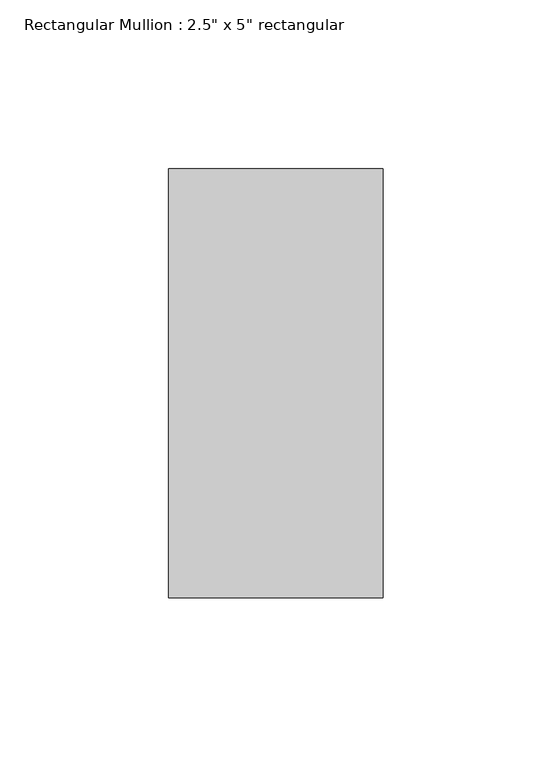
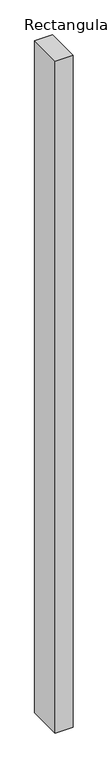
"""IFC4 building model written with IfcOpenShell, lengths in millimetres: member geometry."""

from ifc_helpers import new_model, si_unit, frame, origin, place, context, project, spatial, polyline, outline, extrude, source, transform, mapped, element, save


def member_2dd96db1(model_context):
    return source(origin(), model_context, "Body", "SweptSolid", [
        extrude(outline(polyline([(0.0, 63.5), (0.0, -63.5), (-63.5, -63.5), (-63.5, 63.5), (0.0, 63.5)])), frame((0.0, 0.0, -2544.2333333), z_axis=(0.0, 0.0, 1.0), x_axis=(1.0, 0.0, 0.0)), (0.0, 0.0, 1.0), 2544.2333333),
    ])


if __name__ == "__main__":
    model = new_model("IFC4")
    model_context = context("Model", 3, world=origin())
    ifc_project = project(units=[si_unit("LENGTHUNIT", "METRE", prefix="MILLI")], contexts=[model_context])
    site = spatial("IfcSite", under=ifc_project)
    building = spatial("IfcBuilding", under=site)
    placement = place(None, origin())
    member_shape = member_2dd96db1(model_context)
    element("IfcMember", 1, ObjectType="Rectangular Mullion : 2.5\" x 5\" rectangular", at=placement, inside=building, context=model_context, shape_type="MappedRepresentation", body=[
        mapped(member_shape, transform((0.0, 0.0, 0.0), x_axis=(1.0, 0.0, 0.0), y_axis=(0.0, 1.0, 0.0), z_axis=(0.0, 0.0, 1.0))),
    ])
    save(model, "model.ifc")

# Revit data of these elements
# Type "Rectangular Mullion : 2.5\" x 5\" rectangular"
#   built-in parameter 1007304 = 0.416667 (stored number, unit not read)
#   built-in parameter 1007301 = 0.104167 (stored number, unit not read)
#   built-in parameter 1007300 = 0.104167 (stored number, unit not read)
# Element 1 (IfcMember, "Rectangular Mullion : 2.5\" x 5\" rectangular")
#   Materials on its faces: "Aluminum"
# Materials
#   "Aluminum": class "Metal", colour RGB 247 247 247, transparency 0, Description = "Aluminum 6061", Cost = 0
